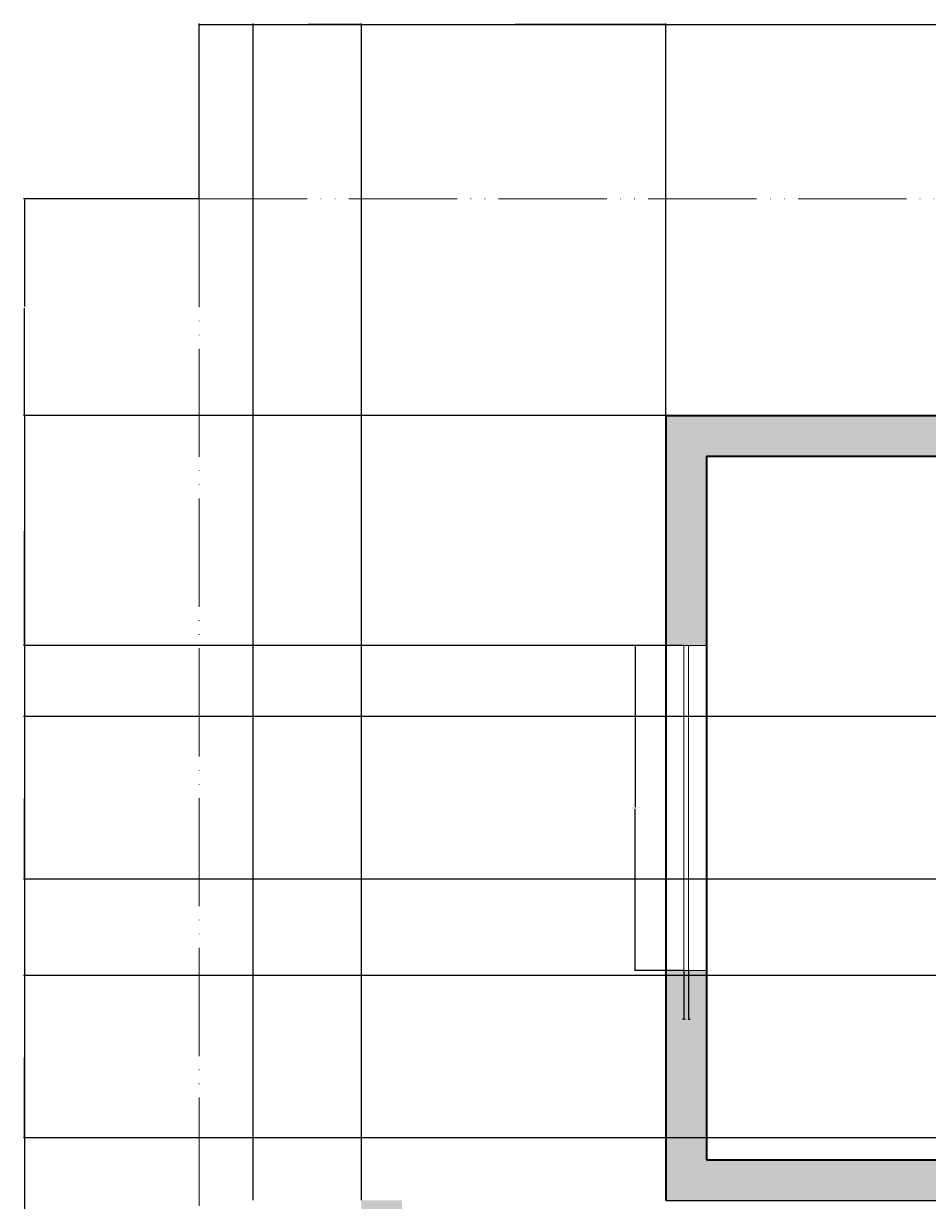
# Model space of a CAD drawing. Units: inches. Extents: x 2847 to 3693, y 1516 to 2098.
# Tile 2 of 6: x 2847 to 3047, y 1837 to 2098. Entities that reach past the tile are written whole.
import ezdxf

# ---------------------------------------------------------------- set-up
doc = ezdxf.new("R2010")
doc.units = ezdxf.units.IN
doc.linetypes.add('ACAD_ISO05W100', pattern=[33, 24, -3, 0, -3, 0, -3])
for name, color, linetype, lineweight in [('A-ANNO-DIMS', 2, 'Continuous', 18), ('A-GLAZ', 4, 'Continuous', 18), ('A-WALL', 7, 'Continuous', 35), ('C-PROP', 7, 'ACAD_ISO05W100', 18)]:
    doc.layers.add(name, color=color, linetype=linetype, lineweight=lineweight)
doc.layers.add('A-WALL-PATT', color=251, linetype='Continuous', lineweight=13, true_color=0x636466)
doc.styles.get("Standard").update_dxf_attribs({"font": 'arial.ttf'})
doc.dimstyles.get("Standard").update_dxf_attribs({"dimtxt": 0.18, "dimasz": 0.18, "dimexe": 0.18, "dimexo": 0.0625, "dimgap": 0.09, "dimtad": 0, "dimtih": 1, "dimtoh": 1, "dimdec": 4, "dimzin": 0, "dimdsep": 46, "dimtxsty": 'Standard', "dimcen": 0.09, "dimadec": 0, "dimazin": 0, "dimtfac": 1, "dimtdec": 4, "dimtofl": 0, "dimtmove": 0, "dimatfit": 3, "dimfxl": 1, "dimtolj": 1, "dimtzin": 0, "dimarcsym": 0})

# ---------------------------------------------------------------- blocks, each defined once
blk = doc.blocks.new('WIN-GLAZ-72IN')
for p, q in [((0, 1), (72, 1)), ((0, 0), (72, 0))]:
    blk.add_line(p, q)
blk = doc.blocks.new('*D13')
at = {"layer": 'A-ANNO-DIMS', "color": 0, "lineweight": -2, "transparency": 16777216}
for p, q in [((2993.28, 1960.12), (2982.37, 1960.12)), ((2982.55, 1959.94), (2982.55, 1924.3)), ((2982.55, 1888.3), (2982.55, 1923.93)), ((2993.28, 1888.12), (2982.37, 1888.12))]:
    blk.add_line(p, q, dxfattribs=at)
at = {"layer": 'A-ANNO-DIMS', "color": 0, "transparency": 16777216}
for points in [[(2982.52, 1959.94), (2982.58, 1959.94), (2982.55, 1960.12)], [(2982.52, 1888.3), (2982.58, 1888.3), (2982.55, 1888.12)]]:
    blk.add_solid(points, dxfattribs=at)
at = {"layer": 'Defpoints', "color": 0, "transparency": 16777216}
for p in [(2993.35, 1960.12), (2982.55, 1888.12), (2993.35, 1888.12)]:
    blk.add_point(p, dxfattribs=at)
at = {"layer": 'A-ANNO-DIMS', "color": 0, "transparency": 16777216, "insert": (2982.55, 1924.12), "char_height": 0.18, "attachment_point": 5}
blk.add_mtext('\\A1;WINDOW 72 TYP.', dxfattribs=at)
blk = doc.blocks.new('*D14')
at = {"layer": 'A-ANNO-DIMS', "color": 0, "lineweight": -2, "transparency": 16777216}
for p, q in [((2993.35, 1888.06), (2993.35, 1877.14)), ((2994.35, 1888.06), (2994.35, 1877.14)), ((2993.17, 1877.32), (2992.99, 1877.32)), ((2994.53, 1877.32), (2994.71, 1877.32))]:
    blk.add_line(p, q, dxfattribs=at)
at = {"layer": 'A-ANNO-DIMS', "color": 0, "transparency": 16777216}
for points in [[(2993.17, 1877.35), (2993.17, 1877.29), (2993.35, 1877.32)], [(2994.53, 1877.35), (2994.53, 1877.29), (2994.35, 1877.32)]]:
    blk.add_solid(points, dxfattribs=at)
at = {"layer": 'Defpoints', "color": 0, "transparency": 16777216}
for p in [(2993.35, 1888.12), (2994.35, 1888.12), (2994.35, 1877.32)]:
    blk.add_point(p, dxfattribs=at)
at = {"layer": 'A-ANNO-DIMS', "color": 0, "transparency": 16777216, "insert": (2993.85, 1877.32), "char_height": 0.18, "attachment_point": 5}
blk.add_mtext('\\A1;1 TYP.', dxfattribs=at)
blk = doc.blocks.new('*D35')
at = {"layer": 'A-ANNO-DIMS', "color": 0, "lineweight": -2, "transparency": 16777216}
for p, q in [((2885.85, 2059.18), (2885.85, 2098)), ((2886.03, 2097.82), (3269.56, 2097.82)), ((3653.67, 2097.82), (3270.13, 2097.82)), ((3653.85, 2059.18), (3653.85, 2098))]:
    blk.add_line(p, q, dxfattribs=at)
at = {"layer": 'A-ANNO-DIMS', "color": 0, "transparency": 16777216}
for points in [[(2886.03, 2097.85), (2886.03, 2097.79), (2885.85, 2097.82)], [(3653.67, 2097.85), (3653.67, 2097.79), (3653.85, 2097.82)]]:
    blk.add_solid(points, dxfattribs=at)
at = {"layer": 'Defpoints', "color": 0, "transparency": 16777216}
for p in [(3653.85, 2097.82), (2885.85, 2059.12), (3653.85, 2059.12)]:
    blk.add_point(p, dxfattribs=at)
at = {"layer": 'A-ANNO-DIMS', "color": 0, "transparency": 16777216, "insert": (3269.85, 2097.82), "char_height": 0.18, "attachment_point": 5}
blk.add_mtext('\\A1;768', dxfattribs=at)
blk = doc.blocks.new('*D38')
at = {"layer": 'A-ANNO-DIMS', "color": 0, "lineweight": -2, "transparency": 16777216}
for p, q in [((2989.283202, 2011.118004), (2846.965702, 2011.118004)), ((2847.145702, 2010.938004), (2847.145702, 1789.298004)), ((2847.145702, 1567.298004), (2847.145702, 1788.938004)), ((2921.783202, 1567.118004), (2846.965702, 1567.118004))]:
    blk.add_line(p, q, dxfattribs=at)
at = {"layer": 'A-ANNO-DIMS', "color": 0, "transparency": 16777216}
for points in [[(2847.115702, 2010.938004), (2847.175702, 2010.938004), (2847.145702, 2011.118004)], [(2847.115702, 1567.298004), (2847.175702, 1567.298004), (2847.145702, 1567.118004)]]:
    blk.add_solid(points, dxfattribs=at)
at = {"layer": 'Defpoints', "color": 0, "transparency": 16777216}
for p in [(2847.145702, 2011.118004), (2989.345702, 2011.118004), (2921.845702, 1567.118004)]:
    blk.add_point(p, dxfattribs=at)
at = {"layer": 'A-ANNO-DIMS', "color": 0, "transparency": 16777216, "insert": (2847.145702, 1789.118004), "char_height": 0.18, "attachment_point": 5}
blk.add_mtext('\\A1;444', dxfattribs=at)
blk = doc.blocks.new('*D39')
at = {"layer": 'A-ANNO-DIMS', "color": 0, "lineweight": -2, "transparency": 16777216}
for p, q in [((2989.35, 2011.18), (2989.35, 2098)), ((2989.53, 2097.82), (3085.71, 2097.82)), ((3182.67, 2097.82), (3086.48, 2097.82)), ((3182.85, 2002.18), (3182.85, 2098))]:
    blk.add_line(p, q, dxfattribs=at)
at = {"layer": 'A-ANNO-DIMS', "color": 0, "transparency": 16777216}
for points in [[(2989.53, 2097.85), (2989.53, 2097.79), (2989.35, 2097.82)], [(3182.67, 2097.85), (3182.67, 2097.79), (3182.85, 2097.82)]]:
    blk.add_solid(points, dxfattribs=at)
at = {"layer": 'Defpoints', "color": 0, "transparency": 16777216}
for p in [(3182.85, 2097.82), (2989.35, 2011.12), (3182.85, 2002.12)]:
    blk.add_point(p, dxfattribs=at)
at = {"layer": 'A-ANNO-DIMS', "color": 0, "transparency": 16777216, "insert": (3086.1, 2097.82), "char_height": 0.18, "attachment_point": 5}
blk.add_mtext('\\A1;193.5', dxfattribs=at)
blk = doc.blocks.new('*D44')
at = {"layer": 'A-ANNO-DIMS', "color": 0, "lineweight": -2, "transparency": 16777216}
for p, q in [((2921.85, 1837.18), (2921.85, 2098)), ((2922.03, 2097.82), (2955.27, 2097.82)), ((2989.17, 2097.82), (2955.92, 2097.82)), ((2989.35, 1837.18), (2989.35, 2098))]:
    blk.add_line(p, q, dxfattribs=at)
at = {"layer": 'A-ANNO-DIMS', "color": 0, "transparency": 16777216}
for points in [[(2922.03, 2097.85), (2922.03, 2097.79), (2921.85, 2097.82)], [(2989.17, 2097.85), (2989.17, 2097.79), (2989.35, 2097.82)]]:
    blk.add_solid(points, dxfattribs=at)
at = {"layer": 'Defpoints', "color": 0, "transparency": 16777216}
for p in [(2989.35, 2097.82), (2921.85, 1837.12), (2989.35, 1837.12)]:
    blk.add_point(p, dxfattribs=at)
at = {"layer": 'A-ANNO-DIMS', "color": 0, "transparency": 16777216, "insert": (2955.6, 2097.82), "char_height": 0.18, "attachment_point": 5}
blk.add_mtext('\\A1;67.5', dxfattribs=at)
blk = doc.blocks.new('*D50')
at = {"layer": 'A-ANNO-DIMS', "color": 0, "lineweight": -2, "transparency": 16777216}
for p, q in [((2989.41, 2011.12), (3692.73, 2011.12)), ((3692.55, 2010.94), (3692.55, 1924.3)), ((3692.55, 1837.3), (3692.55, 1923.94)), ((2989.41, 1837.12), (3692.73, 1837.12))]:
    blk.add_line(p, q, dxfattribs=at)
at = {"layer": 'A-ANNO-DIMS', "color": 0, "transparency": 16777216}
for points in [[(3692.52, 2010.94), (3692.58, 2010.94), (3692.55, 2011.12)], [(3692.52, 1837.3), (3692.58, 1837.3), (3692.55, 1837.12)]]:
    blk.add_solid(points, dxfattribs=at)
at = {"layer": 'Defpoints', "color": 0, "transparency": 16777216}
for p in [(2989.35, 2011.12), (3692.55, 2011.12), (2989.35, 1837.12)]:
    blk.add_point(p, dxfattribs=at)
at = {"layer": 'A-ANNO-DIMS', "color": 0, "transparency": 16777216, "insert": (3692.55, 1924.12), "char_height": 0.18, "attachment_point": 5}
blk.add_mtext('\\A1;174', dxfattribs=at)
blk = doc.blocks.new('*D55')
at = {"layer": 'A-ANNO-DIMS', "color": 0, "lineweight": -2, "transparency": 16777216}
for p, q in [((3178.28, 1944.37), (2846.97, 1944.37)), ((2847.15, 1944.19), (2847.15, 1926.55)), ((2847.15, 1908.55), (2847.15, 1926.19)), ((3178.28, 1908.37), (2846.97, 1908.37))]:
    blk.add_line(p, q, dxfattribs=at)
at = {"layer": 'A-ANNO-DIMS', "color": 0, "transparency": 16777216}
for points in [[(2847.12, 1944.19), (2847.18, 1944.19), (2847.15, 1944.37)], [(2847.12, 1908.55), (2847.18, 1908.55), (2847.15, 1908.37)]]:
    blk.add_solid(points, dxfattribs=at)
at = {"layer": 'Defpoints', "color": 0, "transparency": 16777216}
for p in [(2847.15, 1944.37), (3178.35, 1944.37), (3178.35, 1908.37)]:
    blk.add_point(p, dxfattribs=at)
at = {"layer": 'A-ANNO-DIMS', "color": 0, "transparency": 16777216, "insert": (2847.15, 1926.37), "char_height": 0.18, "attachment_point": 5}
blk.add_mtext('\\A1;36', dxfattribs=at)
blk = doc.blocks.new('*D61')
at = {"layer": 'A-ANNO-DIMS', "color": 0, "lineweight": -2, "transparency": 16777216}
for p, q in [((2885.78, 2059.12), (2846.97, 2059.12)), ((2847.15, 2058.94), (2847.15, 2035.3)), ((2847.15, 2011.3), (2847.15, 2034.94)), ((2989.28, 2011.12), (2846.97, 2011.12))]:
    blk.add_line(p, q, dxfattribs=at)
at = {"layer": 'A-ANNO-DIMS', "color": 0, "transparency": 16777216}
for points in [[(2847.12, 2058.94), (2847.18, 2058.94), (2847.15, 2059.12)], [(2847.12, 2011.3), (2847.18, 2011.3), (2847.15, 2011.12)]]:
    blk.add_solid(points, dxfattribs=at)
at = {"layer": 'Defpoints', "color": 0, "transparency": 16777216}
for p in [(2847.15, 2059.12), (2885.85, 2059.12), (2989.35, 2011.12)]:
    blk.add_point(p, dxfattribs=at)
at = {"layer": 'A-ANNO-DIMS', "color": 0, "transparency": 16777216, "insert": (2847.15, 2035.12), "char_height": 0.18, "attachment_point": 5}
blk.add_mtext('\\A1;48', dxfattribs=at)
blk = doc.blocks.new('*D63')
at = {"layer": 'A-ANNO-DIMS', "color": 0, "lineweight": -2, "transparency": 16777216}
for p, q in [((2897.85, 1837.18), (2897.85, 2098)), ((2898.03, 2097.82), (2909.63, 2097.82)), ((2921.67, 2097.82), (2910.07, 2097.82)), ((2921.85, 1837.18), (2921.85, 2098))]:
    blk.add_line(p, q, dxfattribs=at)
at = {"layer": 'A-ANNO-DIMS', "color": 0, "transparency": 16777216}
for points in [[(2898.03, 2097.85), (2898.03, 2097.79), (2897.85, 2097.82)], [(2921.67, 2097.85), (2921.67, 2097.79), (2921.85, 2097.82)]]:
    blk.add_solid(points, dxfattribs=at)
at = {"layer": 'Defpoints', "color": 0, "transparency": 16777216}
for p in [(2921.85, 2097.82), (2897.85, 1837.12), (2921.85, 1837.12)]:
    blk.add_point(p, dxfattribs=at)
at = {"layer": 'A-ANNO-DIMS', "color": 0, "transparency": 16777216, "insert": (2909.85, 2097.82), "char_height": 0.18, "attachment_point": 5}
blk.add_mtext('\\A1;24', dxfattribs=at)
blk = doc.blocks.new('*D65')
at = {"layer": 'A-ANNO-DIMS', "color": 0, "lineweight": -2, "transparency": 16777216}
for p, q in [((2989.28, 2011.12), (2846.97, 2011.12)), ((2847.15, 2010.94), (2847.15, 1985.8)), ((2847.15, 1960.3), (2847.15, 1985.44)), ((2989.28, 1960.12), (2846.97, 1960.12))]:
    blk.add_line(p, q, dxfattribs=at)
at = {"layer": 'A-ANNO-DIMS', "color": 0, "transparency": 16777216}
for points in [[(2847.12, 2010.94), (2847.18, 2010.94), (2847.15, 2011.12)], [(2847.12, 1960.3), (2847.18, 1960.3), (2847.15, 1960.12)]]:
    blk.add_solid(points, dxfattribs=at)
at = {"layer": 'Defpoints', "color": 0, "transparency": 16777216}
for p in [(2847.15, 2011.12), (2989.35, 2011.12), (2989.35, 1960.12)]:
    blk.add_point(p, dxfattribs=at)
at = {"layer": 'A-ANNO-DIMS', "color": 0, "transparency": 16777216, "insert": (2847.15, 1985.62), "char_height": 0.18, "attachment_point": 5}
blk.add_mtext('\\A1;51', dxfattribs=at)
blk = doc.blocks.new('*D74')
at = {"layer": 'A-ANNO-DIMS', "color": 0, "lineweight": -2, "transparency": 16777216}
for p, q in [((3182.78, 1886.99), (2846.97, 1886.99)), ((2847.15, 1886.81), (2847.15, 1869.17)), ((2847.15, 1851.17), (2847.15, 1868.81)), ((3182.78, 1850.99), (2846.97, 1850.99))]:
    blk.add_line(p, q, dxfattribs=at)
at = {"layer": 'A-ANNO-DIMS', "color": 0, "transparency": 16777216}
for points in [[(2847.12, 1886.81), (2847.18, 1886.81), (2847.15, 1886.99)], [(2847.12, 1851.17), (2847.18, 1851.17), (2847.15, 1850.99)]]:
    blk.add_solid(points, dxfattribs=at)
at = {"layer": 'Defpoints', "color": 0, "transparency": 16777216}
for p in [(3182.85, 1886.99), (2847.15, 1850.99), (3182.85, 1850.99)]:
    blk.add_point(p, dxfattribs=at)
at = {"layer": 'A-ANNO-DIMS', "color": 0, "transparency": 16777216, "insert": (2847.15, 1868.99), "char_height": 0.18, "attachment_point": 5}
blk.add_mtext('\\A1;36', dxfattribs=at)

msp = doc.modelspace()

# ---------------------------------------------------------------- hatches: boundary and pattern name
at = {"layer": 'A-WALL-PATT'}
h = msp.add_hatch(color=256, dxfattribs=at)
h.dxf.hatch_style = 1
h.paths.add_polyline_path([(2998.3457, 2002.118), (3178.3457, 2002.118), (3178.3457, 1944.368, -0.0341147), (3182.8457, 1944.4698), (3182.8457, 2002.118), (3200.8457, 2002.118), (3200.8457, 2011.118), (2989.3457, 2011.118), (2989.3457, 1960.118), (2998.3457, 1960.118)])
h.paths.add_polyline_path([(2998.3457, 1888.118), (2989.3457, 1888.118), (2989.3457, 1837.118), (3089.8457, 1837.118), (3089.8457, 1778.618), (3098.8457, 1778.618), (3098.8457, 1837.118), (3130.3457, 1837.118, -0.05293254), (3130.1282, 1846.118), (2998.3457, 1846.118)])
h.paths.add_polyline_path([(3263.8457, 2002.118), (3311.8457, 2002.118), (3311.8457, 2011.118), (3263.8457, 2011.118), (3236.8457, 2011.118), (3236.8457, 2002.118), (3254.8457, 2002.118), (3254.8457, 1908.368), (3182.8457, 1908.368), (3178.3457, 1908.368), (3178.3457, 1886.993), (3182.8457, 1886.993), (3182.8457, 1903.868), (3254.8457, 1903.868), (3254.8457, 1846.118), (3182.8457, 1846.118), (3182.8457, 1850.993), (3178.3457, 1850.993), (3178.3457, 1837.118), (3254.8457, 1837.118), (3254.8457, 1790.618), (3263.8457, 1790.618), (3263.8457, 1837.118)])
h.paths.add_polyline_path([(2930.8457, 1837.118), (2921.8457, 1837.118), (2921.8457, 1828.118), (2930.8457, 1828.118)])
h.paths.add_polyline_path([(2930.8457, 1600.118), (2921.8457, 1600.118), (2921.8457, 1591.118), (2930.8457, 1591.118)])
h.paths.add_polyline_path([(3098.8457, 1658.618), (3089.8457, 1658.618), (3089.8457, 1591.118), (3140.8457, 1591.118), (3140.8457, 1600.118), (3098.8457, 1600.118)])
h.paths.add_polyline_path([(3305.8457, 1600.118), (3263.8457, 1600.118), (3263.8457, 1646.618), (3254.8457, 1646.618), (3254.8457, 1600.118), (3212.8457, 1600.118), (3212.8457, 1591.118), (3254.8457, 1591.118), (3305.8457, 1591.118)])
h.paths.add_polyline_path([(3470.8457, 1600.118), (3428.8457, 1600.118), (3428.8457, 1756.118), (3430.26, 1756.118), (3430.26, 1765.118), (3428.8457, 1765.118), (3419.8457, 1765.118), (3419.8457, 1600.118), (3377.8457, 1600.118), (3377.8457, 1591.118), (3470.8457, 1591.118)])
h.paths.add_polyline_path([(3593.8457, 1642.118), (3584.8457, 1642.118), (3584.8457, 1600.118), (3542.8457, 1600.118), (3542.8457, 1591.118), (3593.8457, 1591.118)])
h.paths.add_polyline_path([(3593.8457, 1796.083), (3584.8457, 1796.083), (3584.8457, 1765.118), (3505.3457, 1765.118), (3505.3457, 1837.118), (3584.8457, 1837.118), (3584.8457, 1832.083), (3593.8457, 1832.083), (3593.8457, 1837.118), (3593.8457, 1924.118), (3584.8457, 1924.118), (3584.8457, 1846.118), (3478.26, 1846.118), (3478.26, 1837.118), (3500.8457, 1837.118), (3500.8457, 1765.118), (3478.26, 1765.118, -0.03536449), (3478.26, 1758.7816), (3478.26, 1756.118), (3584.8457, 1756.118), (3584.8457, 1714.118), (3593.8457, 1714.118)])
h.paths.add_polyline_path([(3593.8457, 2011.118), (3536.8457, 2011.118), (3536.8457, 2002.118), (3584.8457, 2002.118), (3584.8457, 1960.118), (3593.8457, 1960.118)])
h.paths.add_polyline_path([(3476.8457, 2011.118), (3371.8457, 2011.118), (3371.8457, 2002.118), (3419.8457, 2002.118), (3419.8457, 1837.118), (3428.8457, 1837.118), (3430.26, 1837.118), (3430.26, 1846.118), (3428.8457, 1846.118), (3428.8457, 2002.118), (3476.8457, 2002.118)])

# ---------------------------------------------------------------- linework, layer by layer
at = {"layer": 'A-GLAZ'}
for p, q in [((2998.3457, 1960.118), (2989.3457, 1960.118)), ((2998.3457, 1888.118), (2989.3457, 1888.118))]:
    msp.add_line(p, q, dxfattribs=at)
at = {"layer": 'A-WALL'}
for p, q in [((2989.3457, 2011.118), (3263.8457, 2011.118)), ((2989.3457, 2011.118), (2989.3457, 1837.118)), ((2998.3457, 2002.118), (3178.3457, 2002.118)), ((2998.3457, 2002.118), (2998.3457, 1846.118)), ((2998.3457, 1846.118), (3130.3457, 1846.118))]:
    msp.add_line(p, q, dxfattribs=at)
at = {"layer": 'C-PROP'}
for q in [(3653.8457, 2059.118), (2885.8457, 1555.118)]:
    msp.add_line((2885.8457, 2059.118), q, dxfattribs=at)

# ---------------------------------------------------------------- block references
at = {"layer": 'A-GLAZ', "rotation": 270}
msp.add_blockref('WIN-GLAZ-72IN', (2993.3457, 1960.1177), dxfattribs=at)

# ---------------------------------------------------------------- dimensions: what is measured, and where the dimension line sits
at = {"layer": 'A-ANNO-DIMS'}
for base, p1, p2, override, picture, middle in [((3653.8457, 2097.818), (2885.8457, 2059.118), (3653.8457, 2059.118), {"dimdec": 0, "dimlfac": 1, "dimrnd": 0, "dimzin": 0, "dimdsep": 46, "dimlunit": 2}, '*D35', (3269.8457, 2097.818)), ((2921.8457, 2097.818), (2897.8457, 1837.118), (2921.8457, 1837.118), {"dimdec": 0, "dimlfac": 1, "dimrnd": 0, "dimzin": 0, "dimdsep": 46, "dimlunit": 2}, '*D63', (2909.8457, 2097.818)), ((2989.3457, 2097.818), (2921.8457, 1837.118), (2989.3457, 1837.118), {"dimdec": 1, "dimlfac": 1, "dimrnd": 0, "dimzin": 0, "dimdsep": 46, "dimlunit": 2}, '*D44', (2955.5957, 2097.818)), ((3182.8457, 2097.818), (2989.3457, 2011.118), (3182.8457, 2002.118), {"dimdec": 1, "dimlfac": 1, "dimrnd": 0, "dimzin": 0, "dimdsep": 46, "dimlunit": 2}, '*D39', (3086.0957, 2097.818))]:
    dim = msp.add_linear_dim(base=base, p1=p1, p2=p2, dimstyle='Standard', override=override, dxfattribs=at)
    dim.commit()
    dim.dimension.update_dxf_attribs({"geometry": picture, "text_midpoint": middle})
for base, p1, p2, picture, middle in [((2847.1457, 2059.118), (2989.3457, 2011.118), (2885.8457, 2059.118), '*D61', (2847.1457, 2035.118)), ((2847.1457, 2011.118), (2921.8457, 1567.118), (2989.3457, 2011.118), '*D38', (2847.1457, 1789.118)), ((2847.1457, 2011.118), (2989.3457, 1960.118), (2989.3457, 2011.118), '*D65', (2847.1457, 1985.618)), ((3692.5457, 2011.118), (2989.3457, 1837.118), (2989.3457, 2011.118), '*D50', (3692.5457, 1924.118)), ((2847.1457, 1944.368), (3178.3457, 1908.368), (3178.3457, 1944.368), '*D55', (2847.1457, 1926.368)), ((2847.1457, 1850.993), (3182.8457, 1886.993), (3182.8457, 1850.993), '*D74', (2847.1457, 1868.993))]:
    dim = msp.add_linear_dim(base=base, p1=p1, p2=p2, angle=90, dimstyle='Standard', override={"dimdec": 0, "dimlfac": 1, "dimrnd": 0, "dimzin": 0, "dimdsep": 46, "dimlunit": 2}, dxfattribs=at)
    dim.commit()
    dim.dimension.update_dxf_attribs({"geometry": picture, "text_midpoint": middle})
dim = msp.add_linear_dim(base=(2982.5457, 1888.118), p1=(2993.3457, 1960.118), p2=(2993.3457, 1888.118), angle=270, text='WINDOW <> TYP.', dimstyle='Standard', override={"dimdec": 0, "dimlfac": 1, "dimrnd": 0, "dimzin": 0, "dimdsep": 46, "dimlunit": 2}, dxfattribs=at)
dim.commit()
dim.dimension.update_dxf_attribs({"geometry": '*D13', "text_midpoint": (2982.5457, 1924.118)})
dim = msp.add_linear_dim(base=(2994.3457, 1877.318), p1=(2993.3457, 1888.118), p2=(2994.3457, 1888.118), text='<> TYP.', dimstyle='Standard', override={"dimdec": 0, "dimlfac": 1, "dimrnd": 0, "dimzin": 0, "dimdsep": 46, "dimlunit": 2}, dxfattribs=at)
dim.commit()
dim.dimension.update_dxf_attribs({"geometry": '*D14', "text_midpoint": (2993.8457, 1877.318)})

doc.saveas('drawing.dxf')
